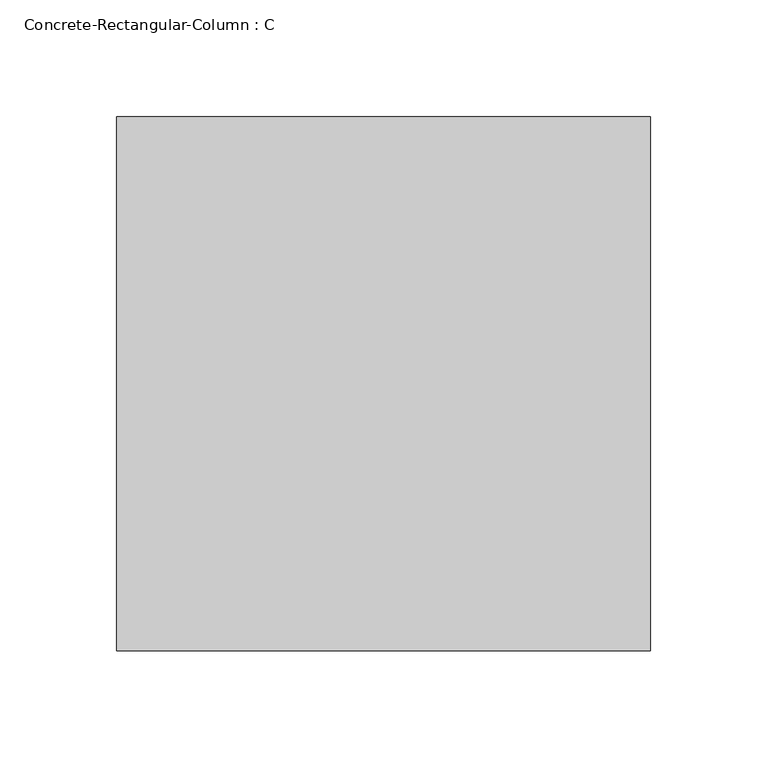
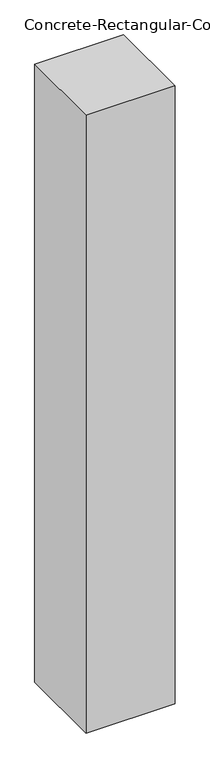
"""IFC4 building model written with IfcOpenShell, lengths in millimetres: column geometry, Concrete-Rectangular-Column : C."""

from ifc_helpers import new_model, si_unit, frame, origin, place, context, project, spatial, polyline, outline, extrude, source, transform, mapped, element, save


def concrete_rectangular_column_c_1fc459bc(model_context):
    return source(origin(), model_context, "Body", "SweptSolid", [
        extrude(outline(polyline([(114.3, 114.3), (114.3, -114.3), (-114.3, -114.3), (-114.3, 114.3), (114.3, 114.3)])), frame((0.0, 0.0, -1676.4), z_axis=(0.0, 0.0, 1.0), x_axis=(1.0, 0.0, 0.0)), (0.0, 0.0, 1.0), 1676.4),
    ])


if __name__ == "__main__":
    model = new_model("IFC4")
    model_context = context("Model", 3, world=origin())
    ifc_project = project(units=[si_unit("LENGTHUNIT", "METRE", prefix="MILLI")], contexts=[model_context])
    site = spatial("IfcSite", under=ifc_project)
    building = spatial("IfcBuilding", under=site)
    placement = place(None, origin())
    concrete_rectangular_column_c_shape = concrete_rectangular_column_c_1fc459bc(model_context)
    element("IfcColumn", 1, ObjectType="Concrete-Rectangular-Column : C", at=placement, inside=building, context=model_context, shape_type="MappedRepresentation", body=[
        mapped(concrete_rectangular_column_c_shape, transform((0.0, 0.0, 0.0), x_axis=(1.0, 0.0, 0.0), y_axis=(0.0, 1.0, 0.0), z_axis=(0.0, 0.0, 1.0))),
    ])
    save(model, "model.ifc")

# Revit data of these elements
# Type "Concrete-Rectangular-Column : C"
#   b = 228.6 mm
#   h = 228.6 mm
#   Structural Material [instance default] = Concrete, Cast-in-Place gray
# Element 1 (IfcColumn, "Concrete-Rectangular-Column : C")
#   Materials on its faces: "Concrete, Cast-in-Place gray"
# Materials
#   "Concrete, Cast-in-Place gray": class "Concrete", colour RGB 192 192 192, transparency 0, Description = "Cast-in-place concrete", Cost = 0
